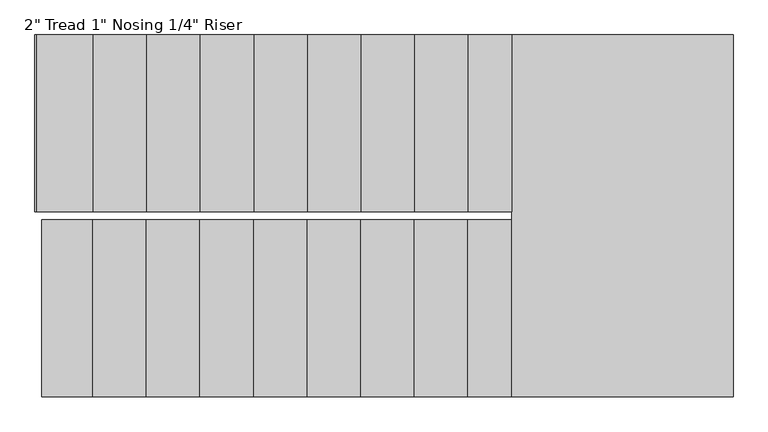
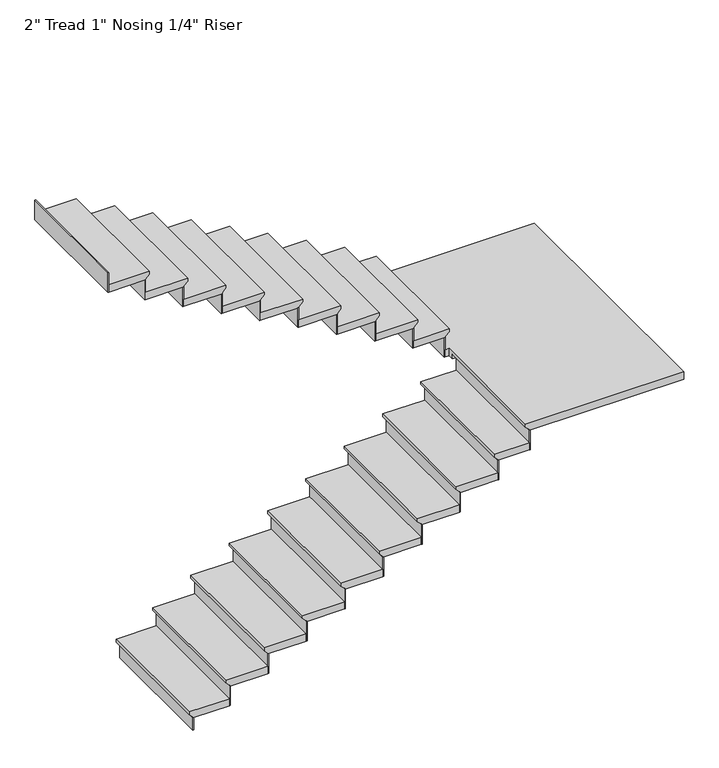
"""IFC4 building model written with IfcOpenShell, lengths in millimetres: stair flight geometry."""

from ifc_helpers import new_model, si_unit, origin, place, context, project, spatial, faceted_brep, source, transform, mapped, element, save


def stair_flight_18d05731(model_context):
    return source(origin(), model_context, "Body", "Brep", [
        faceted_brep([(-1903.1876145, -1606.0595056, 118.11), (-1903.1876145, -1606.0595056, 137.16), (-1903.1876145, -767.8595056, 137.16), (-1903.1876145, -767.8595056, 118.11), (-1877.7876145, -1606.0595056, 92.71), (-1877.7876145, -767.8595056, 92.71), (-1635.543606, -1606.0595056, 137.16), (-1635.543606, -767.8595056, 137.16), (-1877.7876145, -767.8595056, 86.36), (-1635.543606, -767.8595056, 86.36), (-1635.543606, -1606.0595056, 86.36), (-1877.7876145, -1606.0595056, 86.36)], [[[0, 1, 2, 3]], [[4, 0, 3, 5]], [[2, 1, 6, 7]], [[8, 9, 10, 11]], [[2, 7, 9, 8, 5, 3]], [[8, 11, 4, 5]], [[6, 1, 0, 4, 11, 10]], [[7, 6, 10, 9]]]),
        faceted_brep([(-1877.7876145, -1606.0595056, 86.36), (-1877.7876145, -1606.0595056, 0.0), (-1871.4376145, -1606.0595056, 0.0), (-1871.4376145, -1606.0595056, 86.36), (-1877.7876145, -767.8595056, 86.36), (-1871.4376145, -767.8595056, 86.36), (-1871.4376145, -767.8595056, 0.0), (-1877.7876145, -767.8595056, 0.0)], [[[0, 1, 2, 3]], [[4, 5, 6, 7]], [[1, 0, 4, 7]], [[2, 1, 7, 6]], [[3, 2, 6, 5]], [[0, 3, 5, 4]]]),
        faceted_brep([(-1635.543606, -1606.0595056, 223.52), (-1635.543606, -1606.0595056, 86.36), (-1629.193606, -1606.0595056, 86.36), (-1629.193606, -1606.0595056, 223.52), (-1635.543606, -767.8595056, 223.52), (-1629.193606, -767.8595056, 223.52), (-1629.193606, -767.8595056, 86.36), (-1635.543606, -767.8595056, 86.36)], [[[0, 1, 2, 3]], [[4, 5, 6, 7]], [[1, 0, 4, 7]], [[2, 1, 7, 6]], [[3, 2, 6, 5]], [[0, 3, 5, 4]]]),
        faceted_brep([(-1660.943606, -767.8595056, 274.32), (-1660.943606, -1606.0595056, 274.32), (-1381.543606, -1606.0595056, 274.32), (-1381.543606, -767.8595056, 274.32), (-1635.543606, -767.8595056, 223.52), (-1381.543606, -767.8595056, 223.52), (-1381.543606, -1606.0595056, 223.52), (-1635.543606, -1606.0595056, 223.52), (-1635.543606, -767.8595056, 229.87), (-1660.943606, -767.8595056, 255.27), (-1635.543606, -1606.0595056, 229.87), (-1660.943606, -1606.0595056, 255.27)], [[[0, 1, 2, 3]], [[4, 5, 6, 7]], [[0, 3, 5, 4, 8, 9]], [[4, 7, 10, 8]], [[2, 1, 11, 10, 7, 6]], [[3, 2, 6, 5]], [[11, 1, 0, 9]], [[10, 11, 9, 8]]]),
        faceted_brep([(-1381.543606, -1606.0595056, 360.68), (-1381.543606, -1606.0595056, 223.52), (-1375.193606, -1606.0595056, 223.52), (-1375.193606, -1606.0595056, 360.68), (-1381.543606, -767.8595056, 360.68), (-1375.193606, -767.8595056, 360.68), (-1375.193606, -767.8595056, 223.52), (-1381.543606, -767.8595056, 223.52)], [[[0, 1, 2, 3]], [[4, 5, 6, 7]], [[1, 0, 4, 7]], [[2, 1, 7, 6]], [[3, 2, 6, 5]], [[0, 3, 5, 4]]]),
        faceted_brep([(-1406.943606, -767.8595056, 411.48), (-1406.943606, -1606.0595056, 411.48), (-1127.543606, -1606.0595056, 411.48), (-1127.543606, -767.8595056, 411.48), (-1381.543606, -767.8595056, 360.68), (-1127.543606, -767.8595056, 360.68), (-1127.543606, -1606.0595056, 360.68), (-1381.543606, -1606.0595056, 360.68), (-1381.543606, -767.8595056, 367.03), (-1406.943606, -767.8595056, 392.43), (-1381.543606, -1606.0595056, 367.03), (-1406.943606, -1606.0595056, 392.43)], [[[0, 1, 2, 3]], [[4, 5, 6, 7]], [[0, 3, 5, 4, 8, 9]], [[4, 7, 10, 8]], [[2, 1, 11, 10, 7, 6]], [[3, 2, 6, 5]], [[11, 1, 0, 9]], [[10, 11, 9, 8]]]),
        faceted_brep([(-1127.543606, -1606.0595056, 497.84), (-1127.543606, -1606.0595056, 360.68), (-1121.193606, -1606.0595056, 360.68), (-1121.193606, -1606.0595056, 497.84), (-1127.543606, -767.8595056, 497.84), (-1121.193606, -767.8595056, 497.84), (-1121.193606, -767.8595056, 360.68), (-1127.543606, -767.8595056, 360.68)], [[[0, 1, 2, 3]], [[4, 5, 6, 7]], [[1, 0, 4, 7]], [[2, 1, 7, 6]], [[3, 2, 6, 5]], [[0, 3, 5, 4]]]),
        faceted_brep([(-1152.943606, -767.8595056, 548.64), (-1152.943606, -1606.0595056, 548.64), (-873.543606, -1606.0595056, 548.64), (-873.543606, -767.8595056, 548.64), (-1127.543606, -767.8595056, 497.84), (-873.543606, -767.8595056, 497.84), (-873.543606, -1606.0595056, 497.84), (-1127.543606, -1606.0595056, 497.84), (-1127.543606, -767.8595056, 504.19), (-1152.943606, -767.8595056, 529.59), (-1127.543606, -1606.0595056, 504.19), (-1152.943606, -1606.0595056, 529.59)], [[[0, 1, 2, 3]], [[4, 5, 6, 7]], [[0, 3, 5, 4, 8, 9]], [[4, 7, 10, 8]], [[2, 1, 11, 10, 7, 6]], [[3, 2, 6, 5]], [[11, 1, 0, 9]], [[10, 11, 9, 8]]]),
        faceted_brep([(-873.543606, -1606.0595056, 635.0), (-873.543606, -1606.0595056, 497.84), (-867.193606, -1606.0595056, 497.84), (-867.193606, -1606.0595056, 635.0), (-873.543606, -767.8595056, 635.0), (-867.193606, -767.8595056, 635.0), (-867.193606, -767.8595056, 497.84), (-873.543606, -767.8595056, 497.84)], [[[0, 1, 2, 3]], [[4, 5, 6, 7]], [[1, 0, 4, 7]], [[2, 1, 7, 6]], [[3, 2, 6, 5]], [[0, 3, 5, 4]]]),
        faceted_brep([(-898.943606, -767.8595056, 685.8), (-898.943606, -1606.0595056, 685.8), (-619.543606, -1606.0595056, 685.8), (-619.543606, -767.8595056, 685.8), (-873.543606, -767.8595056, 635.0), (-619.543606, -767.8595056, 635.0), (-619.543606, -1606.0595056, 635.0), (-873.543606, -1606.0595056, 635.0), (-873.543606, -767.8595056, 641.35), (-898.943606, -767.8595056, 666.75), (-873.543606, -1606.0595056, 641.35), (-898.943606, -1606.0595056, 666.75)], [[[0, 1, 2, 3]], [[4, 5, 6, 7]], [[0, 3, 5, 4, 8, 9]], [[4, 7, 10, 8]], [[2, 1, 11, 10, 7, 6]], [[3, 2, 6, 5]], [[11, 1, 0, 9]], [[10, 11, 9, 8]]]),
        faceted_brep([(-619.543606, -1606.0595056, 772.16), (-619.543606, -1606.0595056, 635.0), (-613.193606, -1606.0595056, 635.0), (-613.193606, -1606.0595056, 772.16), (-619.543606, -767.8595056, 772.16), (-613.193606, -767.8595056, 772.16), (-613.193606, -767.8595056, 635.0), (-619.543606, -767.8595056, 635.0)], [[[0, 1, 2, 3]], [[4, 5, 6, 7]], [[1, 0, 4, 7]], [[2, 1, 7, 6]], [[3, 2, 6, 5]], [[0, 3, 5, 4]]]),
        faceted_brep([(-644.943606, -767.8595056, 822.96), (-644.943606, -1606.0595056, 822.96), (-365.543606, -1606.0595056, 822.96), (-365.543606, -767.8595056, 822.96), (-619.543606, -767.8595056, 772.16), (-365.543606, -767.8595056, 772.16), (-365.543606, -1606.0595056, 772.16), (-619.543606, -1606.0595056, 772.16), (-619.543606, -767.8595056, 778.51), (-644.943606, -767.8595056, 803.91), (-619.543606, -1606.0595056, 778.51), (-644.943606, -1606.0595056, 803.91)], [[[0, 1, 2, 3]], [[4, 5, 6, 7]], [[0, 3, 5, 4, 8, 9]], [[4, 7, 10, 8]], [[2, 1, 11, 10, 7, 6]], [[3, 2, 6, 5]], [[11, 1, 0, 9]], [[10, 11, 9, 8]]]),
        faceted_brep([(-365.543606, -1606.0595056, 909.32), (-365.543606, -1606.0595056, 772.16), (-359.193606, -1606.0595056, 772.16), (-359.193606, -1606.0595056, 909.32), (-365.543606, -767.8595056, 909.32), (-359.193606, -767.8595056, 909.32), (-359.193606, -767.8595056, 772.16), (-365.543606, -767.8595056, 772.16)], [[[0, 1, 2, 3]], [[4, 5, 6, 7]], [[1, 0, 4, 7]], [[2, 1, 7, 6]], [[3, 2, 6, 5]], [[0, 3, 5, 4]]]),
        faceted_brep([(-390.943606, -767.8595056, 960.12), (-390.943606, -1606.0595056, 960.12), (-111.543606, -1606.0595056, 960.12), (-111.543606, -767.8595056, 960.12), (-365.543606, -767.8595056, 909.32), (-111.543606, -767.8595056, 909.32), (-111.543606, -1606.0595056, 909.32), (-365.543606, -1606.0595056, 909.32), (-365.543606, -767.8595056, 915.67), (-390.943606, -767.8595056, 941.07), (-365.543606, -1606.0595056, 915.67), (-390.943606, -1606.0595056, 941.07)], [[[0, 1, 2, 3]], [[4, 5, 6, 7]], [[0, 3, 5, 4, 8, 9]], [[4, 7, 10, 8]], [[2, 1, 11, 10, 7, 6]], [[3, 2, 6, 5]], [[11, 1, 0, 9]], [[10, 11, 9, 8]]]),
        faceted_brep([(-111.543606, -1606.0595056, 1046.48), (-111.543606, -1606.0595056, 909.32), (-105.193606, -1606.0595056, 909.32), (-105.193606, -1606.0595056, 1046.48), (-111.543606, -767.8595056, 1046.48), (-105.193606, -767.8595056, 1046.48), (-105.193606, -767.8595056, 909.32), (-111.543606, -767.8595056, 909.32)], [[[0, 1, 2, 3]], [[4, 5, 6, 7]], [[1, 0, 4, 7]], [[2, 1, 7, 6]], [[3, 2, 6, 5]], [[0, 3, 5, 4]]]),
        faceted_brep([(-136.943606, -767.8595056, 1097.28), (-136.943606, -1606.0595056, 1097.28), (142.456394, -1606.0595056, 1097.28), (142.456394, -767.8595056, 1097.28), (-111.543606, -767.8595056, 1046.48), (142.456394, -767.8595056, 1046.48), (142.456394, -1606.0595056, 1046.48), (-111.543606, -1606.0595056, 1046.48), (-111.543606, -767.8595056, 1052.83), (-136.943606, -767.8595056, 1078.23), (-111.543606, -1606.0595056, 1052.83), (-136.943606, -1606.0595056, 1078.23)], [[[0, 1, 2, 3]], [[4, 5, 6, 7]], [[0, 3, 5, 4, 8, 9]], [[4, 7, 10, 8]], [[2, 1, 11, 10, 7, 6]], [[3, 2, 6, 5]], [[11, 1, 0, 9]], [[10, 11, 9, 8]]]),
        faceted_brep([(142.456394, -1606.0595056, 1183.64), (142.456394, -1606.0595056, 1046.48), (148.806394, -1606.0595056, 1046.48), (148.806394, -1606.0595056, 1183.64), (142.456394, -767.8595056, 1183.64), (148.806394, -767.8595056, 1183.64), (148.806394, -767.8595056, 1046.48), (142.456394, -767.8595056, 1046.48)], [[[0, 1, 2, 3]], [[4, 5, 6, 7]], [[1, 0, 4, 7]], [[2, 1, 7, 6]], [[3, 2, 6, 5]], [[0, 3, 5, 4]]]),
        faceted_brep([(117.056394, -767.8595056, 1234.44), (117.056394, -1606.0595056, 1234.44), (350.8830625, -1606.0595056, 1234.44), (350.8830625, -767.8595056, 1234.44), (142.456394, -767.8595056, 1183.64), (350.8830625, -767.8595056, 1183.64), (350.8830625, -1606.0595056, 1183.64), (142.456394, -1606.0595056, 1183.64), (142.456394, -767.8595056, 1189.99), (117.056394, -767.8595056, 1215.39), (142.456394, -1606.0595056, 1189.99), (117.056394, -1606.0595056, 1215.39)], [[[0, 1, 2, 3]], [[4, 5, 6, 7]], [[0, 3, 5, 4, 8, 9]], [[4, 7, 10, 8]], [[2, 1, 11, 10, 7, 6]], [[3, 2, 6, 5]], [[11, 1, 0, 9]], [[10, 11, 9, 8]]]),
        faceted_brep([(350.8830625, -1606.0595056, 1320.8), (350.8830625, -1606.0595056, 1183.64), (357.2330625, -1606.0595056, 1183.64), (357.2330625, -1606.0595056, 1320.8), (350.8830625, -767.8595056, 1320.8), (357.2330625, -767.8595056, 1320.8), (357.2330625, -767.8595056, 1183.64), (350.8830625, -767.8595056, 1183.64)], [[[0, 1, 2, 3]], [[4, 5, 6, 7]], [[1, 0, 4, 7]], [[2, 1, 7, 6]], [[3, 2, 6, 5]], [[0, 3, 5, 4]]]),
        faceted_brep([(300.0830625, -729.7595056, 1371.6), (325.4830625, -729.7595056, 1371.6), (325.4830625, -1606.0595056, 1371.6), (1373.4123855, -1606.0595056, 1371.6), (1373.4123855, 108.4404944, 1371.6), (300.0830625, 108.4404944, 1371.6), (325.4830625, -729.7595056, 1320.8), (300.0830625, -729.7595056, 1320.8), (300.0830625, 108.4404944, 1320.8), (1373.4123855, 108.4404944, 1320.8), (1373.4123855, -1606.0595056, 1320.8), (350.8830625, -1606.0595056, 1320.8), (350.8830625, -767.8595056, 1320.8), (325.4830625, -767.8595056, 1320.8), (325.4830625, -767.8595056, 1352.55), (325.4830625, -1606.0595056, 1352.55), (350.8830625, -767.8595056, 1327.15), (350.8830625, -1606.0595056, 1327.15)], [[[0, 1, 2, 3, 4, 5]], [[6, 7, 8, 9, 10, 11, 12, 13]], [[1, 0, 7, 6]], [[2, 1, 6, 13, 14, 15]], [[13, 12, 16, 14]], [[12, 11, 17, 16]], [[3, 2, 15, 17, 11, 10]], [[4, 3, 10, 9]], [[5, 4, 9, 8]], [[0, 5, 8, 7]], [[17, 15, 14, 16]]]),
        faceted_brep([(300.0830625, 108.4404944, 1457.96), (300.0830625, 108.4404944, 1320.8), (293.7330625, 108.4404944, 1320.8), (293.7330625, 108.4404944, 1457.96), (300.0830625, -729.7595056, 1457.96), (293.7330625, -729.7595056, 1457.96), (293.7330625, -729.7595056, 1320.8), (300.0830625, -729.7595056, 1320.8)], [[[0, 1, 2, 3]], [[4, 5, 6, 7]], [[1, 0, 4, 7]], [[2, 1, 7, 6]], [[3, 2, 6, 5]], [[0, 3, 5, 4]]]),
        faceted_brep([(325.4830625, -729.7595056, 1508.76), (325.4830625, 108.4404944, 1508.76), (91.656394, 108.4404944, 1508.76), (91.656394, -729.7595056, 1508.76), (300.0830625, -729.7595056, 1457.96), (91.656394, -729.7595056, 1457.96), (91.656394, 108.4404944, 1457.96), (300.0830625, 108.4404944, 1457.96), (300.0830625, -729.7595056, 1464.31), (325.4830625, -729.7595056, 1489.71), (300.0830625, 108.4404944, 1464.31), (325.4830625, 108.4404944, 1489.71)], [[[0, 1, 2, 3]], [[4, 5, 6, 7]], [[0, 3, 5, 4, 8, 9]], [[4, 7, 10, 8]], [[2, 1, 11, 10, 7, 6]], [[3, 2, 6, 5]], [[11, 1, 0, 9]], [[10, 11, 9, 8]]]),
        faceted_brep([(91.656394, 108.4404944, 1595.12), (91.656394, 108.4404944, 1457.96), (85.306394, 108.4404944, 1457.96), (85.306394, 108.4404944, 1595.12), (91.656394, -729.7595056, 1595.12), (85.306394, -729.7595056, 1595.12), (85.306394, -729.7595056, 1457.96), (91.656394, -729.7595056, 1457.96)], [[[0, 1, 2, 3]], [[4, 5, 6, 7]], [[1, 0, 4, 7]], [[2, 1, 7, 6]], [[3, 2, 6, 5]], [[0, 3, 5, 4]]]),
        faceted_brep([(117.056394, -729.7595056, 1645.92), (117.056394, 108.4404944, 1645.92), (-162.343606, 108.4404944, 1645.92), (-162.343606, -729.7595056, 1645.92), (91.656394, -729.7595056, 1595.12), (-162.343606, -729.7595056, 1595.12), (-162.343606, 108.4404944, 1595.12), (91.656394, 108.4404944, 1595.12), (91.656394, -729.7595056, 1601.47), (117.056394, -729.7595056, 1626.87), (91.656394, 108.4404944, 1601.47), (117.056394, 108.4404944, 1626.87)], [[[0, 1, 2, 3]], [[4, 5, 6, 7]], [[0, 3, 5, 4, 8, 9]], [[4, 7, 10, 8]], [[2, 1, 11, 10, 7, 6]], [[3, 2, 6, 5]], [[11, 1, 0, 9]], [[10, 11, 9, 8]]]),
        faceted_brep([(-162.343606, 108.4404944, 1732.28), (-162.343606, 108.4404944, 1595.12), (-168.693606, 108.4404944, 1595.12), (-168.693606, 108.4404944, 1732.28), (-162.343606, -729.7595056, 1732.28), (-168.693606, -729.7595056, 1732.28), (-168.693606, -729.7595056, 1595.12), (-162.343606, -729.7595056, 1595.12)], [[[0, 1, 2, 3]], [[4, 5, 6, 7]], [[1, 0, 4, 7]], [[2, 1, 7, 6]], [[3, 2, 6, 5]], [[0, 3, 5, 4]]]),
        faceted_brep([(-136.943606, -729.7595056, 1783.08), (-136.943606, 108.4404944, 1783.08), (-416.343606, 108.4404944, 1783.08), (-416.343606, -729.7595056, 1783.08), (-162.343606, -729.7595056, 1732.28), (-416.343606, -729.7595056, 1732.28), (-416.343606, 108.4404944, 1732.28), (-162.343606, 108.4404944, 1732.28), (-162.343606, -729.7595056, 1738.63), (-136.943606, -729.7595056, 1764.03), (-162.343606, 108.4404944, 1738.63), (-136.943606, 108.4404944, 1764.03)], [[[0, 1, 2, 3]], [[4, 5, 6, 7]], [[0, 3, 5, 4, 8, 9]], [[4, 7, 10, 8]], [[2, 1, 11, 10, 7, 6]], [[3, 2, 6, 5]], [[11, 1, 0, 9]], [[10, 11, 9, 8]]]),
        faceted_brep([(-416.343606, 108.4404944, 1869.44), (-416.343606, 108.4404944, 1732.28), (-422.693606, 108.4404944, 1732.28), (-422.693606, 108.4404944, 1869.44), (-416.343606, -729.7595056, 1869.44), (-422.693606, -729.7595056, 1869.44), (-422.693606, -729.7595056, 1732.28), (-416.343606, -729.7595056, 1732.28)], [[[0, 1, 2, 3]], [[4, 5, 6, 7]], [[1, 0, 4, 7]], [[2, 1, 7, 6]], [[3, 2, 6, 5]], [[0, 3, 5, 4]]]),
        faceted_brep([(-390.943606, -729.7595056, 1920.24), (-390.943606, 108.4404944, 1920.24), (-670.343606, 108.4404944, 1920.24), (-670.343606, -729.7595056, 1920.24), (-416.343606, -729.7595056, 1869.44), (-670.343606, -729.7595056, 1869.44), (-670.343606, 108.4404944, 1869.44), (-416.343606, 108.4404944, 1869.44), (-416.343606, -729.7595056, 1875.79), (-390.943606, -729.7595056, 1901.19), (-416.343606, 108.4404944, 1875.79), (-390.943606, 108.4404944, 1901.19)], [[[0, 1, 2, 3]], [[4, 5, 6, 7]], [[0, 3, 5, 4, 8, 9]], [[4, 7, 10, 8]], [[2, 1, 11, 10, 7, 6]], [[3, 2, 6, 5]], [[11, 1, 0, 9]], [[10, 11, 9, 8]]]),
        faceted_brep([(-670.343606, 108.4404944, 2006.6), (-670.343606, 108.4404944, 1869.44), (-676.693606, 108.4404944, 1869.44), (-676.693606, 108.4404944, 2006.6), (-670.343606, -729.7595056, 2006.6), (-676.693606, -729.7595056, 2006.6), (-676.693606, -729.7595056, 1869.44), (-670.343606, -729.7595056, 1869.44)], [[[0, 1, 2, 3]], [[4, 5, 6, 7]], [[1, 0, 4, 7]], [[2, 1, 7, 6]], [[3, 2, 6, 5]], [[0, 3, 5, 4]]]),
        faceted_brep([(-644.943606, -729.7595056, 2057.4), (-644.943606, 108.4404944, 2057.4), (-924.343606, 108.4404944, 2057.4), (-924.343606, -729.7595056, 2057.4), (-670.343606, -729.7595056, 2006.6), (-924.343606, -729.7595056, 2006.6), (-924.343606, 108.4404944, 2006.6), (-670.343606, 108.4404944, 2006.6), (-670.343606, -729.7595056, 2012.95), (-644.943606, -729.7595056, 2038.35), (-670.343606, 108.4404944, 2012.95), (-644.943606, 108.4404944, 2038.35)], [[[0, 1, 2, 3]], [[4, 5, 6, 7]], [[0, 3, 5, 4, 8, 9]], [[4, 7, 10, 8]], [[2, 1, 11, 10, 7, 6]], [[3, 2, 6, 5]], [[11, 1, 0, 9]], [[10, 11, 9, 8]]]),
        faceted_brep([(-924.343606, 108.4404944, 2143.76), (-924.343606, 108.4404944, 2006.6), (-930.693606, 108.4404944, 2006.6), (-930.693606, 108.4404944, 2143.76), (-924.343606, -729.7595056, 2143.76), (-930.693606, -729.7595056, 2143.76), (-930.693606, -729.7595056, 2006.6), (-924.343606, -729.7595056, 2006.6)], [[[0, 1, 2, 3]], [[4, 5, 6, 7]], [[1, 0, 4, 7]], [[2, 1, 7, 6]], [[3, 2, 6, 5]], [[0, 3, 5, 4]]]),
        faceted_brep([(-898.943606, -729.7595056, 2194.56), (-898.943606, 108.4404944, 2194.56), (-1178.343606, 108.4404944, 2194.56), (-1178.343606, -729.7595056, 2194.56), (-924.343606, -729.7595056, 2143.76), (-1178.343606, -729.7595056, 2143.76), (-1178.343606, 108.4404944, 2143.76), (-924.343606, 108.4404944, 2143.76), (-924.343606, -729.7595056, 2150.11), (-898.943606, -729.7595056, 2175.51), (-924.343606, 108.4404944, 2150.11), (-898.943606, 108.4404944, 2175.51)], [[[0, 1, 2, 3]], [[4, 5, 6, 7]], [[0, 3, 5, 4, 8, 9]], [[4, 7, 10, 8]], [[2, 1, 11, 10, 7, 6]], [[3, 2, 6, 5]], [[11, 1, 0, 9]], [[10, 11, 9, 8]]]),
        faceted_brep([(-1178.343606, 108.4404944, 2280.92), (-1178.343606, 108.4404944, 2143.76), (-1184.693606, 108.4404944, 2143.76), (-1184.693606, 108.4404944, 2280.92), (-1178.343606, -729.7595056, 2280.92), (-1184.693606, -729.7595056, 2280.92), (-1184.693606, -729.7595056, 2143.76), (-1178.343606, -729.7595056, 2143.76)], [[[0, 1, 2, 3]], [[4, 5, 6, 7]], [[1, 0, 4, 7]], [[2, 1, 7, 6]], [[3, 2, 6, 5]], [[0, 3, 5, 4]]]),
        faceted_brep([(-1152.943606, -729.7595056, 2331.72), (-1152.943606, 108.4404944, 2331.72), (-1432.343606, 108.4404944, 2331.72), (-1432.343606, -729.7595056, 2331.72), (-1178.343606, -729.7595056, 2280.92), (-1432.343606, -729.7595056, 2280.92), (-1432.343606, 108.4404944, 2280.92), (-1178.343606, 108.4404944, 2280.92), (-1178.343606, -729.7595056, 2287.27), (-1152.943606, -729.7595056, 2312.67), (-1178.343606, 108.4404944, 2287.27), (-1152.943606, 108.4404944, 2312.67)], [[[0, 1, 2, 3]], [[4, 5, 6, 7]], [[0, 3, 5, 4, 8, 9]], [[4, 7, 10, 8]], [[2, 1, 11, 10, 7, 6]], [[3, 2, 6, 5]], [[11, 1, 0, 9]], [[10, 11, 9, 8]]]),
        faceted_brep([(-1432.343606, 108.4404944, 2418.08), (-1432.343606, 108.4404944, 2280.92), (-1438.693606, 108.4404944, 2280.92), (-1438.693606, 108.4404944, 2418.08), (-1432.343606, -729.7595056, 2418.08), (-1438.693606, -729.7595056, 2418.08), (-1438.693606, -729.7595056, 2280.92), (-1432.343606, -729.7595056, 2280.92)], [[[0, 1, 2, 3]], [[4, 5, 6, 7]], [[1, 0, 4, 7]], [[2, 1, 7, 6]], [[3, 2, 6, 5]], [[0, 3, 5, 4]]]),
        faceted_brep([(-1406.943606, -729.7595056, 2468.88), (-1406.943606, 108.4404944, 2468.88), (-1686.343606, 108.4404944, 2468.88), (-1686.343606, -729.7595056, 2468.88), (-1432.343606, -729.7595056, 2418.08), (-1686.343606, -729.7595056, 2418.08), (-1686.343606, 108.4404944, 2418.08), (-1432.343606, 108.4404944, 2418.08), (-1432.343606, -729.7595056, 2424.43), (-1406.943606, -729.7595056, 2449.83), (-1432.343606, 108.4404944, 2424.43), (-1406.943606, 108.4404944, 2449.83)], [[[0, 1, 2, 3]], [[4, 5, 6, 7]], [[0, 3, 5, 4, 8, 9]], [[4, 7, 10, 8]], [[2, 1, 11, 10, 7, 6]], [[3, 2, 6, 5]], [[11, 1, 0, 9]], [[10, 11, 9, 8]]]),
        faceted_brep([(-1686.343606, 108.4404944, 2555.24), (-1686.343606, 108.4404944, 2418.08), (-1692.693606, 108.4404944, 2418.08), (-1692.693606, 108.4404944, 2555.24), (-1686.343606, -729.7595056, 2555.24), (-1692.693606, -729.7595056, 2555.24), (-1692.693606, -729.7595056, 2418.08), (-1686.343606, -729.7595056, 2418.08)], [[[0, 1, 2, 3]], [[4, 5, 6, 7]], [[1, 0, 4, 7]], [[2, 1, 7, 6]], [[3, 2, 6, 5]], [[0, 3, 5, 4]]]),
        faceted_brep([(-1928.5876145, 108.4404944, 2692.4), (-1928.5876145, 108.4404944, 2555.24), (-1934.9376145, 108.4404944, 2555.24), (-1934.9376145, 108.4404944, 2692.4), (-1928.5876145, -729.7595056, 2692.4), (-1934.9376145, -729.7595056, 2692.4), (-1934.9376145, -729.7595056, 2555.24), (-1928.5876145, -729.7595056, 2555.24)], [[[0, 1, 2, 3]], [[4, 5, 6, 7]], [[1, 0, 4, 7]], [[2, 1, 7, 6]], [[3, 2, 6, 5]], [[0, 3, 5, 4]]]),
        faceted_brep([(-1660.943606, -729.7595056, 2606.04), (-1660.943606, 108.4404944, 2606.04), (-1928.5876145, 108.4404944, 2606.04), (-1928.5876145, -729.7595056, 2606.04), (-1686.343606, -729.7595056, 2555.24), (-1928.5876145, -729.7595056, 2555.24), (-1928.5876145, 108.4404944, 2555.24), (-1686.343606, 108.4404944, 2555.24), (-1686.343606, -729.7595056, 2561.59), (-1660.943606, -729.7595056, 2586.99), (-1686.343606, 108.4404944, 2561.59), (-1660.943606, 108.4404944, 2586.99)], [[[0, 1, 2, 3]], [[4, 5, 6, 7]], [[0, 3, 5, 4, 8, 9]], [[4, 7, 10, 8]], [[2, 1, 11, 10, 7, 6]], [[3, 2, 6, 5]], [[11, 1, 0, 9]], [[10, 11, 9, 8]]]),
    ])


if __name__ == "__main__":
    model = new_model("IFC4")
    model_context = context("Model", 3, world=origin())
    ifc_project = project(units=[si_unit("LENGTHUNIT", "METRE", prefix="MILLI")], contexts=[model_context])
    site = spatial("IfcSite", under=ifc_project)
    building = spatial("IfcBuilding", under=site)
    placement = place(None, origin())
    stair_flight_shape = stair_flight_18d05731(model_context)
    element("IfcStairFlight", 1, ObjectType="2\" Tread 1\" Nosing 1/4\" Riser", at=placement, inside=building, context=model_context, shape_type="MappedRepresentation", body=[
        mapped(stair_flight_shape, transform((0.0, 0.0, 0.0), x_axis=(1.0, 0.0, 0.0), y_axis=(0.0, 1.0, 0.0), z_axis=(0.0, 0.0, 1.0))),
    ])
    save(model, "model.ifc")
